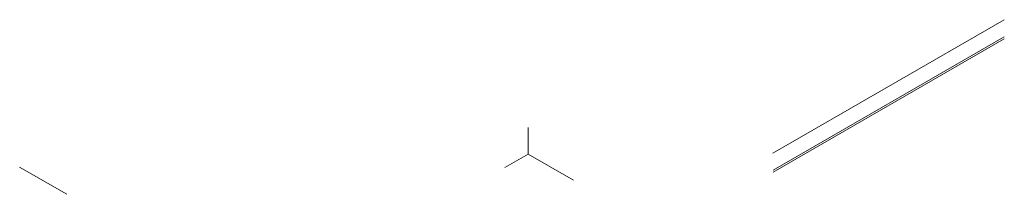
# Model space of a CAD drawing. Units: metres. Extents: x 6326 to 12764, y 4147 to 8354.
# Tile 2 of 2: x 12656 to 12764, y 8335 to 8354. Entities that reach past the tile are written whole.
import ezdxf

# ---------------------------------------------------------------- set-up
doc = ezdxf.new("R2010")
doc.units = ezdxf.units.M
doc.layers.add('A-CONS', color=9, linetype='Continuous', lineweight=13)

msp = doc.modelspace()

# ---------------------------------------------------------------- linework, layer by layer
at = {"layer": 'A-CONS'}
for p, q in [((12738.78, 8339.45), (12764.32, 8354.19)), ((12738.81, 8337.57), (12764.35, 8352.32)), ((12738.81, 8337.35), (12764.35, 8352.09)), ((12711.76, 8342.3), (12711.76, 8339.37)), ((12709.18, 8337.88), (12711.76, 8339.37)), ((12711.76, 8339.37), (12716.77, 8336.48)), ((12655.58, 8337.93), (12660.78, 8334.93))]:
    msp.add_line(p, q, dxfattribs=at)

doc.saveas('drawing.dxf')
